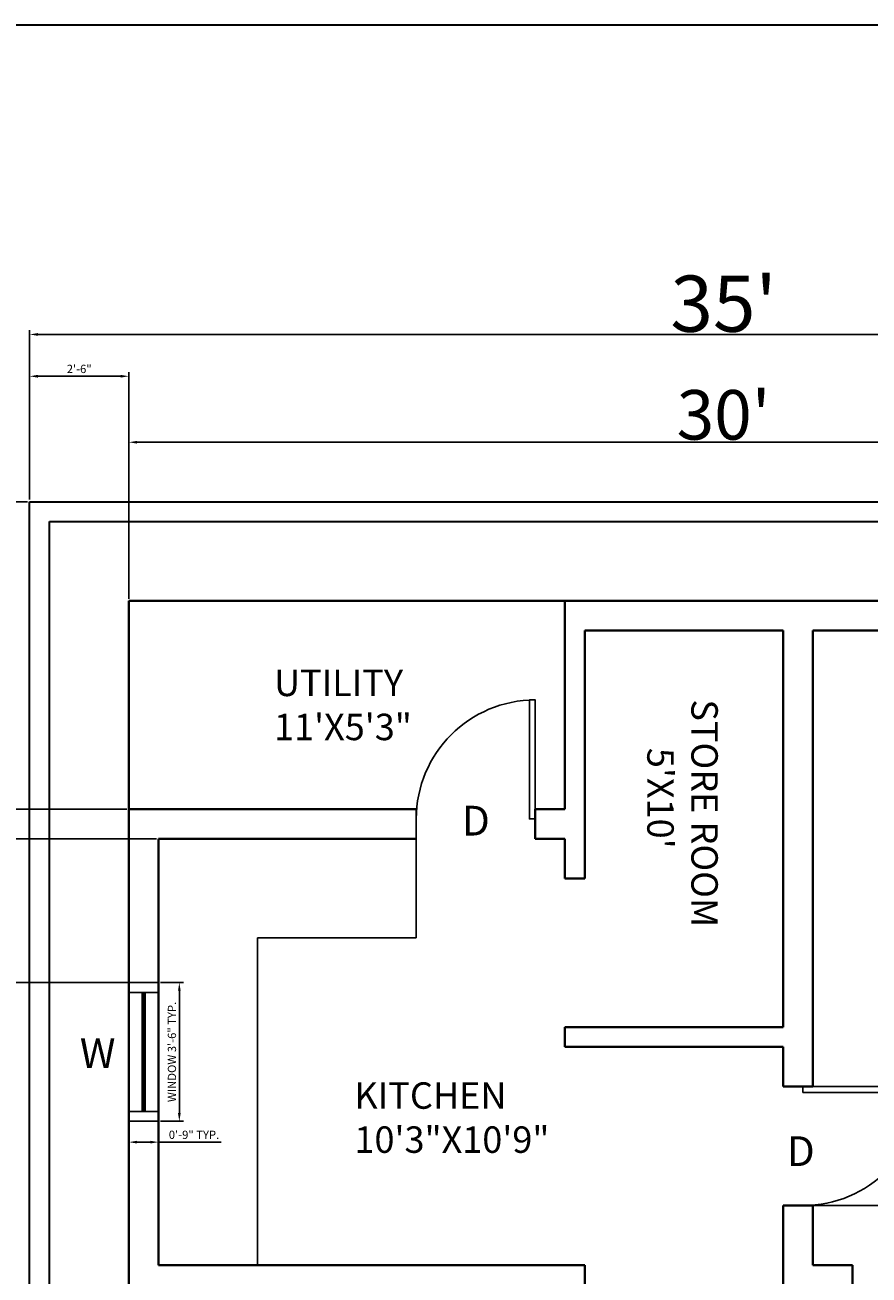
# Model space of a CAD drawing. Units: inches. Extents: x 6038 to 7543, y 3772 to 5131.
# Tile 8 of 14: x 6290 to 6545, y 4753 to 5131. Entities that reach past the tile are written whole.
import ezdxf

# ---------------------------------------------------------------- set-up
doc = ezdxf.new("R2010")
doc.units = ezdxf.units.IN
for name, color, linetype, lineweight in [('A-ANNO-DIMS', 4, 'Continuous', 18), ('A-ANNO-TEXT', 7, 'Continuous', 18), ('A-ANNO-TTLB', 1, 'Continuous', 35), ('A-AREA-IDEN', 2, 'Continuous', 18), ('A-DOOR', 3, 'Continuous', 25), ('A-FLOR-FIXT', 8, 'Continuous', 25), ('A-WALL', 7, 'Continuous', 40)]:
    doc.layers.add(name, color=color, linetype=linetype, lineweight=lineweight)
doc.layers.add('A-GLAZ', color=30, linetype='Continuous', lineweight=25, true_color=0xf26722)
doc.layers.add('C-PROP-WALL', color=251, linetype='Continuous', lineweight=35, true_color=0x636466)
doc.styles.get("Standard").update_dxf_attribs({"font": 'arial.ttf'})
doc.dimstyles.new('ISO-25', dxfattribs={"dimtxt": 2.5, "dimasz": 2.5, "dimexe": 1.25, "dimexo": 0.625, "dimtad": 1, "dimdec": 0, "dimlunit": 3, "dimtxsty": 'Standard', "dimcen": 2.5, "dimadec": 0, "dimazin": 0, "dimtfac": 1, "dimtdec": 0, "dimtmove": 0, "dimatfit": 3, "dimfxl": 1, "dimarcsym": 0})

# ---------------------------------------------------------------- blocks, each defined once
blk = doc.blocks.new('*U7')
for p, q in [((0, 0), (0, -6)), ((-36, 0), (-36, -6))]:
    blk.add_line(p, q)
blk.add_lwpolyline([(0, 0), (0, 36), (-1.75, 36), (-1.75, 0)], close=True)
blk.add_arc((0, 0), 36, 90, 180)
blk = doc.blocks.new('*U9')
for p, q in [((0, 0), (0, -6)), ((36, 0), (36, -6))]:
    blk.add_line(p, q)
blk.add_lwpolyline([(0, 0), (0, 36), (1.75, 36), (1.75, 0)], close=True)
blk.add_arc((0, 0), 36, 0, 90)
blk = doc.blocks.new('*D13')
at = {"layer": 'A-ANNO-DIMS', "color": 0, "lineweight": -2, "transparency": 16777216}
for p, q in [((6321.42, 4957.24), (6321.42, 5005.85)), ((6323.92, 5004.6), (6678.92, 5004.6)), ((6681.42, 4957.24), (6681.42, 5005.85))]:
    blk.add_line(p, q, dxfattribs=at)
at = {"layer": 'A-ANNO-DIMS', "color": 0, "transparency": 16777216}
for points in [[(6323.92, 5005.02), (6323.92, 5004.19), (6321.42, 5004.6)], [(6678.92, 5005.02), (6678.92, 5004.19), (6681.42, 5004.6)]]:
    blk.add_solid(points, dxfattribs=at)
at = {"layer": 'Defpoints', "color": 0, "transparency": 16777216}
for p in [(6681.42, 5004.6), (6321.42, 4956.62), (6681.42, 4956.62)]:
    blk.add_point(p, dxfattribs=at)
at = {"layer": 'A-ANNO-DIMS', "color": 0, "transparency": 16777216, "insert": (6501.42, 5012.89), "char_height": 2.5, "attachment_point": 5}
blk.add_mtext("{\\H6x;30'}", dxfattribs=at)
blk = doc.blocks.new('*D15')
at = {"layer": 'A-ANNO-DIMS', "color": 0, "lineweight": -2, "transparency": 16777216}
for p, q in [((6320.79, 4893.62), (6264.12, 4893.62)), ((6265.37, 4891.12), (6265.37, 4551.12)), ((6320.79, 4548.62), (6264.12, 4548.62))]:
    blk.add_line(p, q, dxfattribs=at)
at = {"layer": 'A-ANNO-DIMS', "color": 0, "transparency": 16777216}
for points in [[(6264.96, 4891.12), (6265.79, 4891.12), (6265.37, 4893.62)], [(6264.96, 4551.12), (6265.79, 4551.12), (6265.37, 4548.62)]]:
    blk.add_solid(points, dxfattribs=at)
at = {"layer": 'Defpoints', "color": 0, "transparency": 16777216}
for p in [(6321.42, 4893.62), (6265.37, 4548.62), (6321.42, 4548.62)]:
    blk.add_point(p, dxfattribs=at)
at = {"layer": 'A-ANNO-DIMS', "color": 0, "transparency": 16777216, "insert": (6257.09, 4721.12), "char_height": 2.5, "attachment_point": 5, "rotation": 90}
blk.add_mtext('{\\H6x;28\'-9"}', dxfattribs=at)
blk = doc.blocks.new('*D16')
at = {"layer": 'A-ANNO-DIMS', "color": 0, "lineweight": -2, "transparency": 16777216}
for p, q in [((6291.42, 4987.24), (6291.42, 5038.47)), ((6711.42, 4987.24), (6711.42, 5038.47)), ((6293.92, 5037.22), (6708.92, 5037.22))]:
    blk.add_line(p, q, dxfattribs=at)
at = {"layer": 'A-ANNO-DIMS', "color": 0, "transparency": 16777216}
for points in [[(6293.92, 5037.63), (6293.92, 5036.8), (6291.42, 5037.22)], [(6708.92, 5037.63), (6708.92, 5036.8), (6711.42, 5037.22)]]:
    blk.add_solid(points, dxfattribs=at)
at = {"layer": 'Defpoints', "color": 0, "transparency": 16777216}
for p in [(6711.42, 5037.22), (6291.42, 4986.62), (6711.42, 4986.62)]:
    blk.add_point(p, dxfattribs=at)
at = {"layer": 'A-ANNO-DIMS', "color": 0, "transparency": 16777216, "insert": (6501.42, 5046.53), "char_height": 2.5, "attachment_point": 5}
blk.add_mtext("{\\H6.8x;35'}", dxfattribs=at)
blk = doc.blocks.new('*D17')
at = {"layer": 'A-ANNO-DIMS', "color": 0, "lineweight": -2, "transparency": 16777216}
for p, q in [((6290.79, 4986.62), (6224.51, 4986.62)), ((6225.76, 4984.12), (6225.76, 4365.12)), ((6290.79, 4362.62), (6224.51, 4362.62))]:
    blk.add_line(p, q, dxfattribs=at)
at = {"layer": 'A-ANNO-DIMS', "color": 0, "transparency": 16777216}
for points in [[(6225.34, 4984.12), (6226.18, 4984.12), (6225.76, 4986.62)], [(6225.34, 4365.12), (6226.18, 4365.12), (6225.76, 4362.62)]]:
    blk.add_solid(points, dxfattribs=at)
at = {"layer": 'Defpoints', "color": 0, "transparency": 16777216}
for p in [(6291.42, 4986.62), (6225.76, 4362.62), (6291.42, 4362.62)]:
    blk.add_point(p, dxfattribs=at)
at = {"layer": 'A-ANNO-DIMS', "color": 0, "transparency": 16777216, "insert": (6216.45, 4674.62), "char_height": 2.5, "attachment_point": 5, "rotation": 90}
blk.add_mtext("{\\H6.8x;52'}", dxfattribs=at)
blk = doc.blocks.new('WIN-36-PLAN')
for p, q in [((9, 42), (0, 42)), ((9, 39), (0, 39)), ((4, 39), (4, 3)), ((4.5, 39), (4.5, 3)), ((5, 39), (5, 3)), ((9, 3), (0, 3)), ((9, 0), (0, 0))]:
    blk.add_line(p, q)
blk = doc.blocks.new('*D32')
at = {"layer": 'A-ANNO-DIMS', "color": 0, "lineweight": -2, "transparency": 16777216}
for p, q in [((6331.04, 4841.12), (6337.97, 4841.12)), ((6336.72, 4801.62), (6336.72, 4838.62)), ((6331.04, 4799.12), (6337.97, 4799.12))]:
    blk.add_line(p, q, dxfattribs=at)
at = {"layer": 'A-ANNO-DIMS', "color": 0, "transparency": 16777216}
for points in [[(6336.3, 4838.62), (6337.13, 4838.62), (6336.72, 4841.12)], [(6336.3, 4801.62), (6337.13, 4801.62), (6336.72, 4799.12)]]:
    blk.add_solid(points, dxfattribs=at)
at = {"layer": 'Defpoints', "color": 0, "transparency": 16777216}
for p in [(6330.42, 4841.12), (6336.72, 4841.12), (6330.42, 4799.12)]:
    blk.add_point(p, dxfattribs=at)
at = {"layer": 'A-ANNO-DIMS', "color": 0, "transparency": 16777216, "insert": (6334.8, 4820.12), "char_height": 2.5, "attachment_point": 5, "rotation": 90}
blk.add_mtext('WINDOW 3\'-6" TYP.', dxfattribs=at)
blk = doc.blocks.new('*D33')
at = {"layer": 'A-ANNO-DIMS', "color": 0, "lineweight": -2, "transparency": 16777216}
for p, q in [((6321.42, 4798.49), (6321.42, 4791.57)), ((6330.42, 4798.49), (6330.42, 4791.57)), ((6323.92, 4792.82), (6327.92, 4792.82)), ((6330.42, 4792.82), (6349.41, 4792.82))]:
    blk.add_line(p, q, dxfattribs=at)
at = {"layer": 'A-ANNO-DIMS', "color": 0, "transparency": 16777216}
for points in [[(6323.92, 4793.24), (6323.92, 4792.4), (6321.42, 4792.82)], [(6327.92, 4793.24), (6327.92, 4792.4), (6330.42, 4792.82)]]:
    blk.add_solid(points, dxfattribs=at)
at = {"layer": 'Defpoints', "color": 0, "transparency": 16777216}
for p in [(6321.42, 4799.12), (6330.42, 4799.12), (6330.42, 4792.82)]:
    blk.add_point(p, dxfattribs=at)
at = {"layer": 'A-ANNO-DIMS', "color": 0, "transparency": 16777216, "insert": (6341.16, 4794.72), "char_height": 2.5, "attachment_point": 5}
blk.add_mtext('0\'-9" TYP.', dxfattribs=at)
blk = doc.blocks.new('*D54')
at = {"layer": 'A-ANNO-DIMS', "color": 0, "lineweight": -2, "transparency": 16777216}
for p, q in [((6291.42, 4987.24), (6291.42, 5025.82)), ((6293.92, 5024.57), (6318.92, 5024.57)), ((6321.42, 4957.24), (6321.42, 5025.82))]:
    blk.add_line(p, q, dxfattribs=at)
at = {"layer": 'A-ANNO-DIMS', "color": 0, "transparency": 16777216}
for points in [[(6293.92, 5024.99), (6293.92, 5024.15), (6291.42, 5024.57)], [(6318.92, 5024.99), (6318.92, 5024.15), (6321.42, 5024.57)]]:
    blk.add_solid(points, dxfattribs=at)
at = {"layer": 'Defpoints', "color": 0, "transparency": 16777216}
for p in [(6321.42, 5024.57), (6291.42, 4986.62), (6321.42, 4956.62)]:
    blk.add_point(p, dxfattribs=at)
at = {"layer": 'A-ANNO-DIMS', "color": 0, "transparency": 16777216, "insert": (6306.42, 5026.47), "char_height": 2.5, "attachment_point": 5}
blk.add_mtext('2\'-6"', dxfattribs=at)
blk = doc.blocks.new('*D58')
at = {"layer": 'A-ANNO-DIMS', "color": 0, "lineweight": -2, "transparency": 16777216}
for p, q in [((6520.04, 4809.62), (6750.62, 4809.62)), ((6749.37, 4807.12), (6749.37, 4776.12)), ((6520.04, 4773.62), (6750.62, 4773.62))]:
    blk.add_line(p, q, dxfattribs=at)
at = {"layer": 'A-ANNO-DIMS', "color": 0, "transparency": 16777216}
for points in [[(6748.95, 4807.12), (6749.78, 4807.12), (6749.37, 4809.62)], [(6748.95, 4776.12), (6749.78, 4776.12), (6749.37, 4773.62)]]:
    blk.add_solid(points, dxfattribs=at)
at = {"layer": 'Defpoints', "color": 0, "transparency": 16777216}
for p in [(6519.42, 4809.62), (6519.42, 4773.62), (6749.37, 4773.62)]:
    blk.add_point(p, dxfattribs=at)
at = {"layer": 'A-ANNO-DIMS', "color": 0, "transparency": 16777216, "insert": (6747.46, 4791.62), "char_height": 2.5, "attachment_point": 5, "rotation": 90}
blk.add_mtext('3\'-0"', dxfattribs=at)
blk = doc.blocks.new('*D62')
at = {"layer": 'A-ANNO-DIMS', "color": 0, "lineweight": -2, "transparency": 16777216}
for p, q in [((6329.79, 4884.62), (6252.22, 4884.62)), ((6253.47, 4843.62), (6253.47, 4882.12)), ((6329.79, 4841.12), (6252.22, 4841.12))]:
    blk.add_line(p, q, dxfattribs=at)
at = {"layer": 'A-ANNO-DIMS', "color": 0, "transparency": 16777216}
for points in [[(6253.05, 4882.12), (6253.88, 4882.12), (6253.47, 4884.62)], [(6253.05, 4843.62), (6253.88, 4843.62), (6253.47, 4841.12)]]:
    blk.add_solid(points, dxfattribs=at)
at = {"layer": 'Defpoints', "color": 0, "transparency": 16777216}
for p in [(6253.47, 4884.62), (6330.42, 4884.62), (6330.42, 4841.12)]:
    blk.add_point(p, dxfattribs=at)
at = {"layer": 'A-ANNO-DIMS', "color": 0, "transparency": 16777216, "insert": (6251.55, 4862.87), "char_height": 2.5, "attachment_point": 5, "rotation": 90}
blk.add_mtext('3\'-7 1/2"', dxfattribs=at)

msp = doc.modelspace()

# ---------------------------------------------------------------- linework, layer by layer
at = {"layer": 'A-ANNO-TTLB'}
msp.add_lwpolyline([(6037.83, 5130.86), (7542.53, 5130.86), (7542.53, 3772.09), (6037.83, 3772.09)], close=True, dxfattribs=at)
at = {"layer": 'A-FLOR-FIXT'}
for p, q in [((6408.42, 4893.62), (6408.42, 4854.62)), ((6360.42, 4755.62), (6360.42, 4854.62)), ((6360.42, 4854.62), (6408.42, 4854.62))]:
    msp.add_line(p, q, dxfattribs=at)
at = {"layer": 'A-WALL'}
for p, q in [((6321.42, 4956.62), (6681.42, 4956.62)), ((6321.42, 4548.62), (6321.42, 4956.62)), ((6453.42, 4956.62), (6453.42, 4893.62)), ((6459.42, 4947.62), (6459.42, 4872.62)), ((6459.42, 4947.62), (6519.42, 4947.62)), ((6519.42, 4947.62), (6519.42, 4827.62)), ((6528.42, 4947.62), (6528.42, 4809.62)), ((6528.42, 4947.62), (6672.42, 4947.62)), ((6321.42, 4893.62), (6408.42, 4893.62)), ((6444.42, 4893.62), (6444.42, 4884.62)), ((6444.42, 4893.62), (6453.42, 4893.62)), ((6330.42, 4884.62), (6408.42, 4884.62)), ((6330.42, 4755.62), (6330.42, 4884.62)), ((6444.42, 4884.62), (6453.42, 4884.62)), ((6453.42, 4884.62), (6453.42, 4872.62)), ((6453.42, 4872.62), (6459.42, 4872.62)), ((6453.42, 4827.62), (6519.42, 4827.62)), ((6453.42, 4827.62), (6453.42, 4821.62)), ((6453.42, 4821.62), (6519.42, 4821.62)), ((6519.42, 4821.62), (6519.42, 4809.62)), ((6519.42, 4809.62), (6528.42, 4809.62)), ((6519.42, 4773.62), (6528.42, 4773.62)), ((6519.42, 4773.62), (6519.42, 4668.62)), ((6528.42, 4773.62), (6528.42, 4755.62)), ((6330.42, 4755.62), (6459.42, 4755.62)), ((6459.42, 4755.62), (6459.42, 4749.62)), ((6528.42, 4755.62), (6540.42, 4755.62)), ((6540.42, 4755.62), (6540.42, 4749.62))]:
    msp.add_line(p, q, dxfattribs=at)
at = {"layer": 'C-PROP-WALL'}
for p, q in [((6291.42, 4986.62), (6711.42, 4986.62)), ((6291.42, 4362.62), (6291.42, 4986.62)), ((6297.42, 4980.62), (6705.42, 4980.62)), ((6297.42, 4368.62), (6297.42, 4980.62))]:
    msp.add_line(p, q, dxfattribs=at)

# ---------------------------------------------------------------- block references
at = {"layer": 'A-DOOR'}
msp.add_blockref('*U7', (6444.42, 4890.62), dxfattribs=at)
at = {"layer": 'A-DOOR', "rotation": 270}
msp.add_blockref('*U9', (6525.42, 4809.62), dxfattribs=at)
at = {"layer": 'A-GLAZ'}
msp.add_blockref('WIN-36-PLAN', (6321.42, 4799.12), dxfattribs=at)

# ---------------------------------------------------------------- texts
at = {"layer": 'A-ANNO-TEXT', "char_height": 9, "attachment_point": 1}
for s, insert in [('D', (6422.23, 4894.6)), ('W', (6306.61, 4824.21)), ('D', (6520.55, 4794.59))]:
    msp.add_mtext_dynamic_manual_height_columns(s, width=212.1416, gutter_width=12.5, heights=[0], dxfattribs=dict(at, insert=insert))
at = {"layer": 'A-AREA-IDEN', "char_height": 8, "attachment_point": 1}
for s, width, insert in [('UTILITY\\P11\'X5\'3"', 299.7399, (6365.37, 4935.79)), ('KITCHEN\\P10\'3"X10\'9"', 466.9103, (6389.71, 4810.92))]:
    msp.add_mtext_dynamic_manual_height_columns(s, width=width, gutter_width=12.5, heights=[0], dxfattribs=dict(at, insert=insert))
at = {"layer": 'A-AREA-IDEN', "insert": (6499.66, 4926.79), "char_height": 8, "attachment_point": 1, "rotation": 270}
msp.add_mtext_dynamic_manual_height_columns("STORE ROOM\\P      5'X10'", width=344.76, gutter_width=12.5, heights=[0], dxfattribs=at)

# ---------------------------------------------------------------- dimensions: what is measured, and where the dimension line sits
at = {"layer": 'A-ANNO-DIMS'}
for base, p1, p2, text, override, picture, middle in [((6711.42, 5037.22), (6291.42, 4986.62), (6711.42, 4986.62), '{\\H6.8x;<>}', {"dimclrd": 0, "dimclre": 0, "dimclrt": 0}, '*D16', (6501.42, 5046.53)), ((6681.42, 5004.6), (6321.42, 4956.62), (6681.42, 4956.62), '{\\H6x;<>}', {"dimclrd": 0, "dimclre": 0, "dimclrt": 0}, '*D13', (6501.42, 5012.89)), ((6330.42, 4792.82), (6321.42, 4799.12), (6330.42, 4799.12), '<> TYP.', {"dimdec": 1, "dimlfac": 1, "dimrnd": 0, "dimzin": 1, "dimdsep": 46, "dimlunit": 4, "dimfrac": 2}, '*D33', (6341.16, 4794.72))]:
    dim = msp.add_linear_dim(base=base, p1=p1, p2=p2, text=text, dimstyle='ISO-25', override=override, dxfattribs=at)
    dim.commit()
    dim.dimension.update_dxf_attribs({"geometry": picture, "text_midpoint": middle})
dim = msp.add_linear_dim(base=(6321.42, 5024.57), p1=(6291.42, 4986.62), p2=(6321.42, 4956.62), dimstyle='ISO-25', override={"dimdec": 1, "dimlfac": 1, "dimrnd": 0, "dimzin": 1, "dimdsep": 46, "dimlunit": 4, "dimfrac": 2}, dxfattribs=at)
dim.commit()
dim.dimension.update_dxf_attribs({"geometry": '*D54', "text_midpoint": (6306.42, 5026.47)})
dim = msp.add_linear_dim(base=(6225.76, 4362.62), p1=(6291.42, 4986.62), p2=(6291.42, 4362.62), angle=90, text='{\\H6.8x;<>}', dimstyle='ISO-25', override={"dimclrd": 0, "dimclre": 0, "dimclrt": 0}, dxfattribs=at)
dim.commit()
dim.dimension.update_dxf_attribs({"geometry": '*D17', "text_midpoint": (6225.76, 4674.62), "dimtype": 160})
for base, p1, p2, text, override, picture, middle in [((6265.37, 4548.62), (6321.42, 4893.62), (6321.42, 4548.62), '{\\H6x;<>}', {"dimclrd": 0, "dimclre": 0, "dimclrt": 0}, '*D15', (6257.09, 4721.12)), ((6336.72, 4841.12), (6330.42, 4799.12), (6330.42, 4841.12), 'WINDOW <> TYP.', {"dimdec": 1, "dimlfac": 1, "dimrnd": 0, "dimzin": 1, "dimdsep": 46, "dimlunit": 4, "dimfrac": 2}, '*D32', (6334.8, 4820.12))]:
    dim = msp.add_linear_dim(base=base, p1=p1, p2=p2, angle=90, text=text, dimstyle='ISO-25', override=override, dxfattribs=at)
    dim.commit()
    dim.dimension.update_dxf_attribs({"geometry": picture, "text_midpoint": middle})
for base, p1, p2, picture, middle in [((6253.47, 4884.62), (6330.42, 4841.12), (6330.42, 4884.62), '*D62', (6251.55, 4862.87)), ((6749.37, 4773.62), (6519.42, 4809.62), (6519.42, 4773.62), '*D58', (6747.46, 4791.62))]:
    dim = msp.add_linear_dim(base=base, p1=p1, p2=p2, angle=90, dimstyle='ISO-25', override={"dimdec": 1, "dimlfac": 1, "dimrnd": 0, "dimzin": 1, "dimdsep": 46, "dimlunit": 4, "dimfrac": 2}, dxfattribs=at)
    dim.commit()
    dim.dimension.update_dxf_attribs({"geometry": picture, "text_midpoint": middle})

doc.saveas('drawing.dxf')
